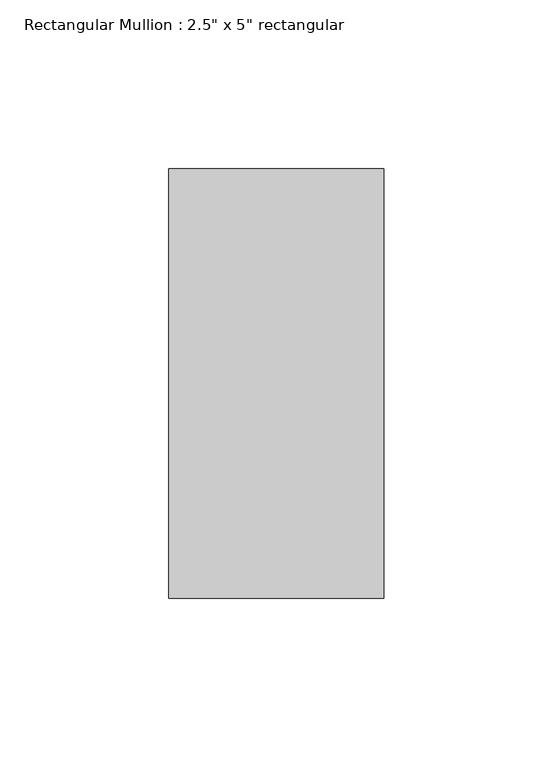
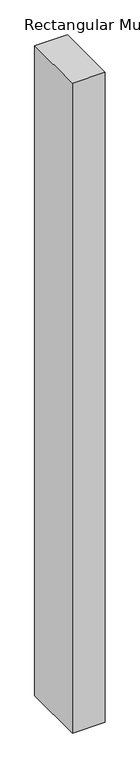
"""IFC4 building model written with IfcOpenShell, lengths in millimetres: member geometry."""

from ifc_helpers import new_model, si_unit, frame, origin, place, context, project, spatial, polyline, outline, extrude, source, transform, mapped, element, save


def member_f32bdbca(model_context):
    return source(origin(), model_context, "Body", "SweptSolid", [
        extrude(outline(polyline([(0.0, 63.5), (0.0, -63.5), (-63.5, -63.5), (-63.5, 63.5), (0.0, 63.5)])), frame((0.0, 0.0, -1333.5), z_axis=(0.0, 0.0, 1.0), x_axis=(1.0, 0.0, 0.0)), (0.0, 0.0, 1.0), 1333.5),
    ])


if __name__ == "__main__":
    model = new_model("IFC4")
    model_context = context("Model", 3, world=origin())
    ifc_project = project(units=[si_unit("LENGTHUNIT", "METRE", prefix="MILLI")], contexts=[model_context])
    site = spatial("IfcSite", under=ifc_project)
    building = spatial("IfcBuilding", under=site)
    placement = place(None, origin())
    member_shape = member_f32bdbca(model_context)
    element("IfcMember", 1, ObjectType="Rectangular Mullion : 2.5\" x 5\" rectangular", at=placement, inside=building, context=model_context, shape_type="MappedRepresentation", body=[
        mapped(member_shape, transform((0.0, 0.0, 0.0), x_axis=(1.0, 0.0, 0.0), y_axis=(0.0, 1.0, 0.0), z_axis=(0.0, 0.0, 1.0))),
    ])
    save(model, "model.ifc")

# Revit data of these elements
# Type "Rectangular Mullion : 2.5\" x 5\" rectangular"
#   built-in parameter 1007304 = 0.416667 (stored number, unit not read)
#   built-in parameter 1007301 = 0.104167 (stored number, unit not read)
#   built-in parameter 1007300 = 0.104167 (stored number, unit not read)
# Element 1 (IfcMember, "Rectangular Mullion : 2.5\" x 5\" rectangular")
#   Materials on its faces: "Aluminum"
# Materials
#   "Aluminum": class "Metal", colour RGB 247 247 247, transparency 0, Description = "Aluminum 6061", Cost = 0
